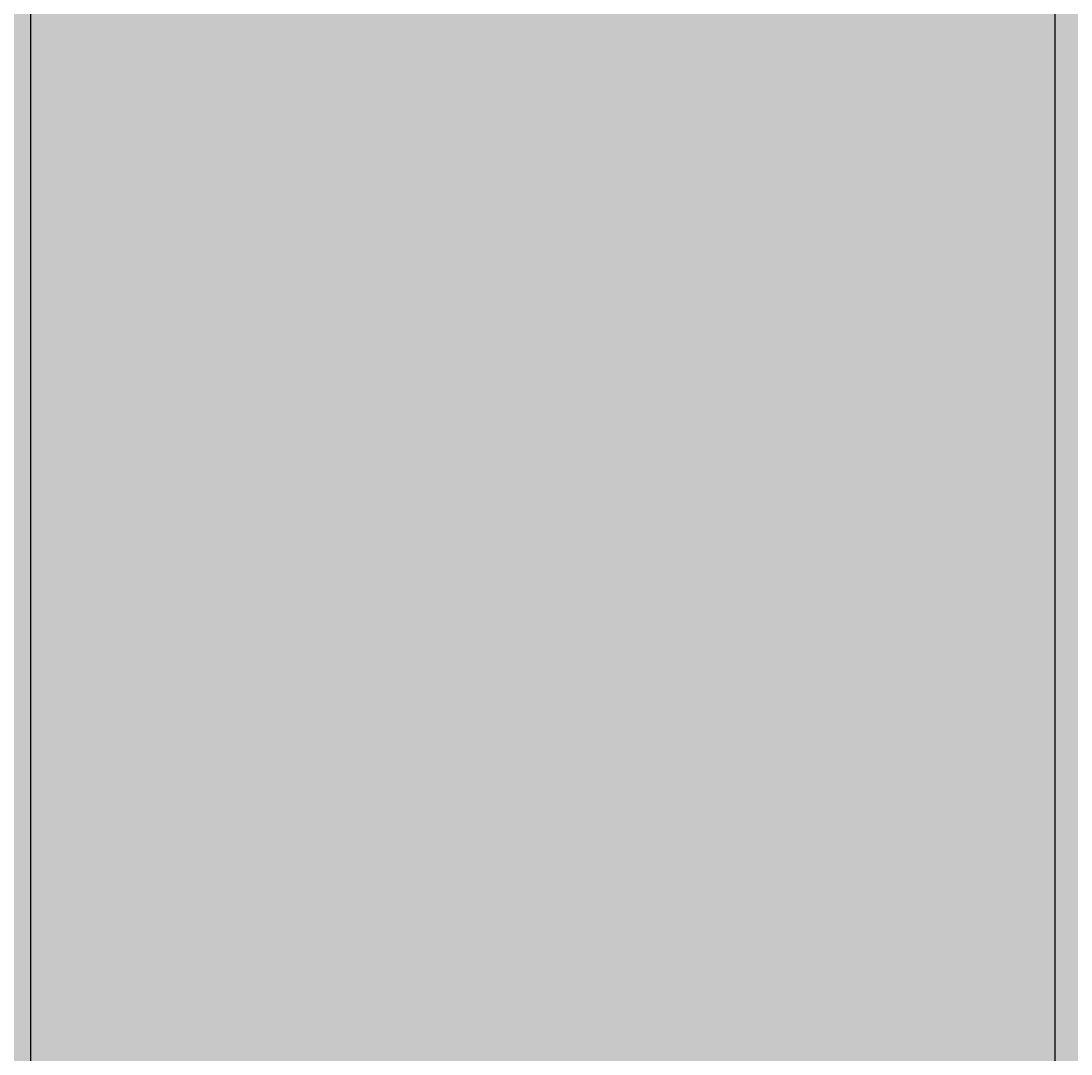
# Model space of a CAD drawing. Units: inches. Extents: x 4508 to 4723, y 847 to 1020.
# Tile 21 of 32: x 4631 to 4657, y 907 to 933. Entities that reach past the tile are written whole.
import ezdxf

# ---------------------------------------------------------------- set-up
doc = ezdxf.new("R2010")
doc.units = ezdxf.units.IN
doc.layers.add('A-ANNO-DIMS', color=2, linetype='Continuous', lineweight=18)
doc.layers.add('A-WALL-PATT', color=254, linetype='Continuous', lineweight=13)
doc.styles.get("Standard").update_dxf_attribs({"font": 'arial.ttf'})
doc.dimstyles.get("Standard").update_dxf_attribs({"dimtxt": 0.18, "dimasz": 0.18, "dimexe": 0.18, "dimexo": 0.0625, "dimgap": 0.09, "dimtad": 0, "dimtih": 1, "dimtoh": 1, "dimdec": 4, "dimzin": 0, "dimdsep": 46, "dimtxsty": 'Standard', "dimcen": 0.09, "dimadec": 0, "dimazin": 0, "dimtfac": 1, "dimtdec": 4, "dimtofl": 0, "dimtmove": 0, "dimatfit": 3, "dimfxl": 1, "dimtolj": 1, "dimtzin": 0, "dimarcsym": 0})

# ---------------------------------------------------------------- blocks, each defined once
blk = doc.blocks.new('*D31')
at = {"layer": 'A-ANNO-DIMS', "color": 0, "lineweight": -2, "transparency": 16777216}
for p, q in [((4630.994, 903.809), (4630.994, 1002.877)), ((4656.994, 903.809), (4656.994, 1002.877)), ((4631.174, 1002.697), (4643.773, 1002.697)), ((4656.814, 1002.697), (4644.214, 1002.697))]:
    blk.add_line(p, q, dxfattribs=at)
at = {"layer": 'A-ANNO-DIMS', "color": 0, "lineweight": 9, "transparency": 16777216}
for points in [[(4631.174, 1002.727), (4631.174, 1002.667), (4630.994, 1002.697)], [(4656.814, 1002.727), (4656.814, 1002.667), (4656.994, 1002.697)]]:
    blk.add_solid(points, dxfattribs=at)
at = {"layer": 'Defpoints', "color": 0, "lineweight": 9, "transparency": 16777216}
for p in [(4656.994, 1002.697), (4630.994, 903.747), (4656.994, 903.747)]:
    blk.add_point(p, dxfattribs=at)
at = {"layer": 'A-ANNO-DIMS', "color": 0, "transparency": 16777216, "insert": (4643.994, 1002.697), "char_height": 0.18, "attachment_point": 5}
blk.add_mtext('\\A1;26', dxfattribs=at)

msp = doc.modelspace()

# ---------------------------------------------------------------- hatches: boundary and pattern name
at = {"layer": 'A-WALL-PATT', "transparency": 33554508}
h = msp.add_hatch(color=256, dxfattribs=at)
h.dxf.hatch_style = 1
h.paths.add_polyline_path([(4661.6706, 954.043, -0.3739004), (4658.5765, 957.6021, -1), (4665.7646, 957.6021, -0.3739004), (4662.6706, 954.043), (4662.6706, 944.4021, -0.2114781), (4670.3062, 945.0869), (4670.3062, 968.0592, -0.4632086), (4663.3246, 973.9783, -0.4632086), (4670.3062, 979.8975), (4670.3062, 994.7469), (4588.9938, 994.7469), (4588.9938, 904.7469), (4657.9938, 904.7469), (4657.9938, 886.7469), (4549.9938, 886.7469), (4549.9938, 878.7469), (4693.9938, 878.7469), (4693.9938, 994.7469), (4671.8062, 994.7469), (4671.8062, 979.4411, -0.2941682), (4675.3246, 973.9783, -0.2941682), (4671.8062, 968.5156), (4671.8062, 944.4278, -0.2741114), (4676.7298, 936.1217, -0.2741114), (4671.8062, 927.8155), (4671.8062, 907.6998, -0.3779645), (4677.0562, 901.7469, -0.3779645), (4671.8062, 895.7939), (4671.8062, 883.7469), (4670.3062, 883.7469), (4670.3062, 895.7939, -0.3779645), (4665.0562, 901.7469, -0.3779645), (4670.3062, 907.6998), (4670.3062, 927.1564, -0.2114781), (4662.6706, 927.8412), (4662.6706, 918.2003, -0.3739004), (4665.7646, 914.6412, -1), (4658.5765, 914.6412, -0.3739004), (4661.6706, 918.2003), (4661.6706, 928.4807, -0.2391825), (4657.7936, 936.1217, -0.2391825), (4661.6706, 943.7626)])

# ---------------------------------------------------------------- dimensions: what is measured, and where the dimension line sits
at = {"layer": 'A-ANNO-DIMS'}
dim = msp.add_linear_dim(base=(4656.9938, 1002.6969), p1=(4630.9938, 903.7469), p2=(4656.9938, 903.7469), dimstyle='Standard', override={"dimdec": 0, "dimlfac": 1, "dimrnd": 0, "dimzin": 0, "dimdsep": 46, "dimlunit": 2}, dxfattribs=at)
dim.commit()
dim.dimension.update_dxf_attribs({"geometry": '*D31', "text_midpoint": (4643.9938, 1002.6969)})

doc.saveas('drawing.dxf')
